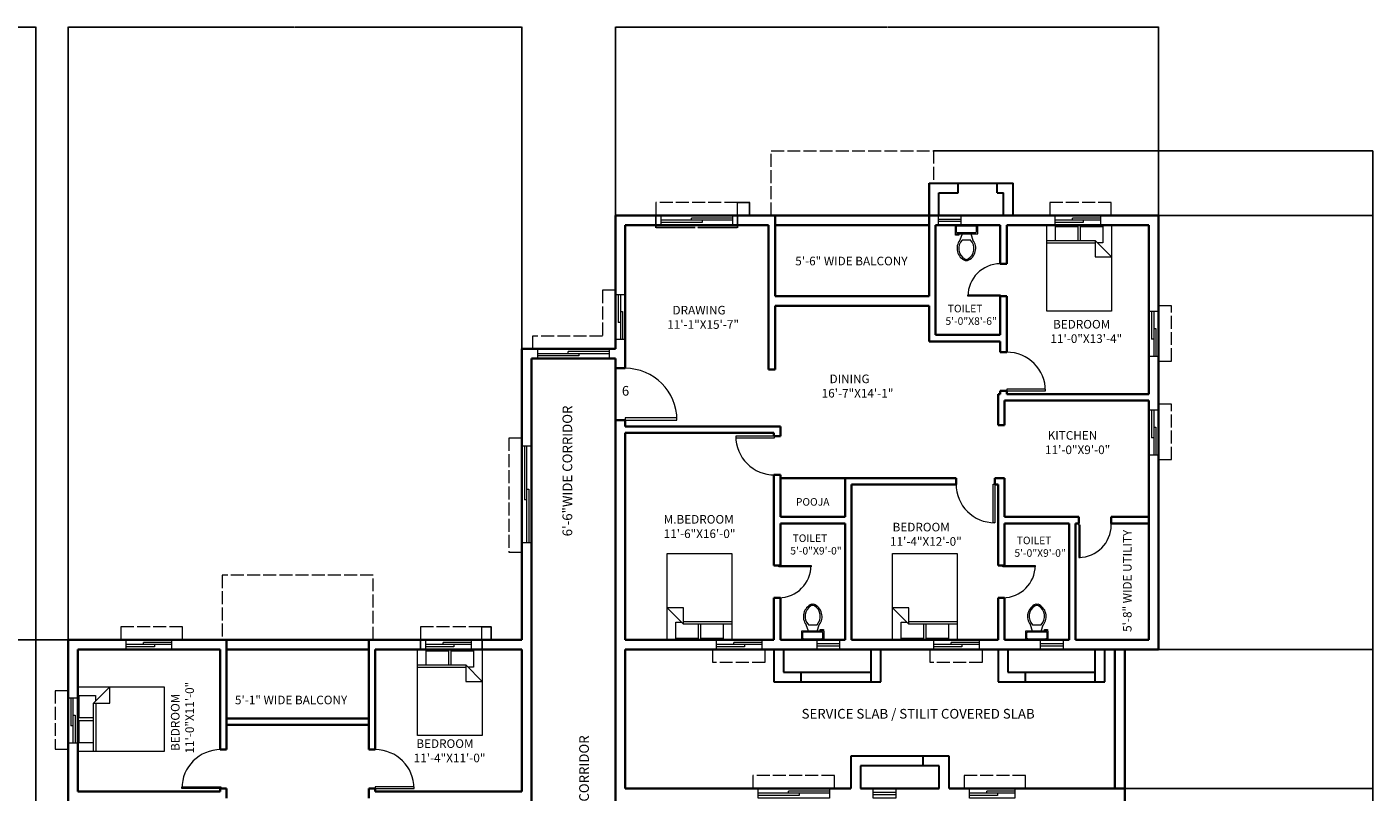
# Model space of a CAD drawing. Units: inches. Extents: x -69 to 2453, y 4803 to 7122.
# Tile 9 of 9: x 1203 to 2453, y 6411 to 7122. Entities that reach past the tile are written whole.
import ezdxf

# ---------------------------------------------------------------- set-up
doc = ezdxf.new("R2010")
doc.units = ezdxf.units.IN
doc.linetypes.add('ACAD_ISO02W100', pattern=[15, 12, -3])
for name, color, linetype, lineweight in [('A-ANNO-DIMS', 2, 'Continuous', 18), ('A-ANNO-IDEN', 2, 'Continuous', 18), ('A-AREA-IDEN', 7, 'Continuous', 18), ('A-DOOR', 3, 'Continuous', 18), ('A-FLOR-FIXT', 9, 'Continuous', 18), ('A-FLOR-OVHD', 8, 'ACAD_ISO02W100', 13), ('A-FURN', 8, 'Continuous', 18), ('A-GLAZ', 244, 'Continuous', 18), ('A-WALL', 7, 'Continuous', 35), ('A-WALL-SRVC', 7, 'Continuous', 30)]:
    doc.layers.add(name, color=color, linetype=linetype, lineweight=lineweight)
doc.styles.get("Standard").update_dxf_attribs({"font": 'arial.ttf'})
doc.dimstyles.get("Standard").update_dxf_attribs({"dimtxt": 0.18, "dimasz": 0.18, "dimexe": 0.18, "dimexo": 0.0625, "dimgap": 0.09, "dimtad": 0, "dimtih": 1, "dimtoh": 1, "dimdec": 4, "dimzin": 0, "dimdsep": 46, "dimtxsty": 'Standard', "dimcen": 0.09, "dimadec": 0, "dimazin": 0, "dimtfac": 1, "dimtdec": 4, "dimtofl": 0, "dimtmove": 0, "dimatfit": 3, "dimfxl": 1, "dimtolj": 1, "dimtzin": 0, "dimarcsym": 0})

# ---------------------------------------------------------------- blocks, each defined once
blk = doc.blocks.new('*U10')
for p, q in [((0, 0), (0, -6)), ((-40, 0), (-40, -6))]:
    blk.add_line(p, q)
blk.add_lwpolyline([(0, 0), (0, 40), (-1.75, 40), (-1.75, 0)], close=True)
blk.add_arc((0, 0), 40, 90, 180)
blk = doc.blocks.new('*U11')
for p, q in [((-40, 0), (-40, 6)), ((0, 0), (0, 6))]:
    blk.add_line(p, q)
blk.add_lwpolyline([(0, 0), (0, -40), (-1.75, -40), (-1.75, 0)], close=True)
blk.add_arc((0, 0), 40, 180, 270)
blk = doc.blocks.new('*U12')
for p, q in [((-40, 0), (-40, -6)), ((0, 0), (0, -6))]:
    blk.add_line(p, q)
blk.add_lwpolyline([(0, 0), (0, 40), (-1.75, 40), (-1.75, 0)], close=True)
blk.add_arc((0, 0), 40, 90, 180)
blk = doc.blocks.new('*U15')
for p, q in [((0, 0), (0, 6)), ((40, 0), (40, 6))]:
    blk.add_line(p, q)
blk.add_lwpolyline([(0, 0), (0, -40), (1.75, -40), (1.75, 0)], close=True)
blk.add_arc((0, 0), 40, 270, 0)
blk = doc.blocks.new('*U13')
for p, q in [((0, 0), (0, -6)), ((40, 0), (40, -6))]:
    blk.add_line(p, q)
blk.add_lwpolyline([(0, 0), (0, 40), (1.75, 40), (1.75, 0)], close=True)
blk.add_arc((0, 0), 40, 0, 90)
blk = doc.blocks.new('*U14')
for p, q in [((0, 0), (0, -6)), ((-40, 0), (-40, -6))]:
    blk.add_line(p, q)
blk.add_lwpolyline([(0, 0), (0, 40), (-1.75, 40), (-1.75, 0)], close=True)
blk.add_arc((0, 0), 40, 90, 180)
blk = doc.blocks.new('Bed - Queen')
for p, q in [((0, -80.00003), (0, 0)), ((0, 0), (59.99999, 0)), ((59.99999, 0), (59.99999, -80.00003)), ((7.99999, -1.2), (28.79998, -1.2)), ((7.99999, -14.4), (7.99999, -1.2)), ((28.79998, -1.2), (28.79998, -14.4)), ((31.19999, -1.2), (51.99999, -1.2)), ((31.19999, -14.4), (31.19999, -1.2)), ((51.99999, -1.2), (51.99999, -16.4)), ((0, -14.4), (44.8, -14.4)), ((44.8, -16.8), (0, -16.8)), ((59.99999, -29.6), (44.8, -14.4)), ((44.8, -14.4), (44.8, -29.6)), ((51.99999, -16.4), (46.79936, -16.4)), ((44.8, -29.6), (59.99999, -29.6)), ((59.99999, -80.00003), (0, -80.00003))]:
    blk.add_line(p, q)
blk = doc.blocks.new('*U33')
for p, q in [((-10, -8.5), (-8, -8.5)), ((-10, -9.5), (-10, -8.5)), ((-7, -9.5), (-10, -9.5)), ((-8, -8.5), (-8, -8)), ((-7, -8), (-7, -9.5)), ((-4, -8), (-6, -14)), ((4, -8), (6, -14)), ((9.5, -6), (9.5, -2)), ((4, -14), (-4, -14))]:
    blk.add_line(p, q)
blk.add_lwpolyline([(10.5, -8), (10.5, 0), (-10.5, 0), (-10.5, -8)], close=True)
for points in [[(-9.5, -2), (-9.5, -6)], [(8.5, -1), (-8.5, -1)], [(-8.5, -7), (8.5, -7)]]:
    blk.add_lwpolyline(points)
for centre, radius, start, end in [((-8.6, -1.9), 0.884, 81.8699, 188.1301), ((-8.6, -6.1), 0.884, 171.8699, 278.1301), ((8.6, -1.9), 0.884, 351.8699, 98.1301), ((8.6, -6.1), 0.884, 261.8699, 8.1301), ((3.5, -21.6), 12.2, 141.4691, 247.9714), ((4.2, -21.8), 11.3, 136.3677, 238.9468), ((-3.5, -21.6), 12.2, 292.0284, 38.5307), ((-4.2, -21.8), 11.3, 301.053, 43.6321), ((0, -27.9), 4, 245.7318, 294.2682), ((0, -29), 4, 254.8605, 285.1395)]:
    blk.add_arc(centre, radius, start, end)
blk = doc.blocks.new('WINDOW-VENT-21IN')
for p, q in [((0, 5.5), (21, 5.5)), ((0, 3.5), (21, 3.5))]:
    blk.add_line(p, q)
blk.add_lwpolyline([(0, 9), (21, 9), (21, 0), (0, 0)], close=True)
blk = doc.blocks.new('WINDOW-SLIDING-42IN')
for p, q in [((2.5, 42), (2.5, 16)), ((4.5, 42), (4.5, 0)), ((4.5, 26), (6.5, 26)), ((6.5, 26), (6.5, 0)), ((4.5, 16), (2.5, 16))]:
    blk.add_line(p, q)
blk.add_lwpolyline([(0, 42), (9, 42), (9, 0), (0, 0)], close=True)
blk = doc.blocks.new('WINDOW-SLIDING-66IN')
for p, q in [((66, 4.5), (0, 4.5)), ((38, 2.5), (0, 2.5)), ((66, 6.5), (28, 6.5)), ((28, 4.5), (28, 6.5)), ((38, 4.5), (38, 2.5))]:
    blk.add_line(p, q)
blk.add_lwpolyline([(66, 9), (66, 0), (0, 0), (0, 9)], close=True)
blk = doc.blocks.new('SUNSHADE-54IN')
for p, q in [((12, 54.3), (0, 54.3)), ((0, 54.3), (0, 0)), ((0, 0), (12, 0))]:
    blk.add_line(p, q)
blk = doc.blocks.new('SUNSHADE-48IN')
for p, q in [((0, 0), (0, 12)), ((48.4, 0), (0, 0)), ((48.4, 12), (48.4, 0))]:
    blk.add_line(p, q)
blk = doc.blocks.new('SUNSHADE-57IN')
for p, q in [((57.1, 12), (0, 12)), ((0, 12), (0, 0)), ((57.1, 0), (57.1, 12))]:
    blk.add_line(p, q)
blk = doc.blocks.new('SUNSHADE-51IN')
for p, q in [((12, 51.4), (0, 51.4)), ((12, 0), (12, 51.4)), ((0, 0), (12, 0))]:
    blk.add_line(p, q)
blk = doc.blocks.new('SUNSHADE-76IN')
for p, q in [((75.7, 12), (0, 12)), ((0, 12), (0, 0)), ((75.7, 0), (75.7, 12))]:
    blk.add_line(p, q)
blk = doc.blocks.new('SERVICE-BAY-78IN')
for p, q in [((0, 30), (78.1, 30)), ((0, 0), (0, 30)), ((27.1, 21), (27.1, 30)), ((63.1, 21), (63.1, 30)), ((78.1, 0), (78.1, 30)), ((9, 0), (9, 21)), ((9, 21), (27.1, 21)), ((63.1, 21), (69.1, 21)), ((69.1, 0), (69.1, 21))]:
    blk.add_line(p, q)
blk = doc.blocks.new('SERVICE-BAY-99IN')
for p, q in [((0, 30), (0, 0)), ((9, 30), (9, 9)), ((90.1, 0), (90.1, 30)), ((99.1, 0), (99.1, 30)), ((0, 0), (99.1, 0)), ((9, 9), (90.1, 9)), ((25.4, 0), (25.4, 9))]:
    blk.add_line(p, q)
blk = doc.blocks.new('*D61')
at = {"layer": 'A-ANNO-DIMS', "color": 0, "lineweight": -2, "transparency": 16777216}
for p, q in [((1568.4, 6552.7), (1568.4, 6544)), ((1625.6, 6552.7), (1625.6, 6544)), ((1568.6, 6544.1), (1595.7, 6544.1)), ((1625.4, 6544.1), (1598.3, 6544.1))]:
    blk.add_line(p, q, dxfattribs=at)
at = {"layer": 'A-ANNO-DIMS', "color": 0, "transparency": 16777216}
for points in [[(1568.6, 6544.2), (1568.6, 6544.1), (1568.4, 6544.1)], [(1625.4, 6544.2), (1625.4, 6544.1), (1625.6, 6544.1)]]:
    blk.add_solid(points, dxfattribs=at)
at = {"layer": 'Defpoints', "color": 0, "transparency": 16777216}
for p in [(1568.4, 6552.7), (1625.6, 6552.7), (1625.6, 6544.1)]:
    blk.add_point(p, dxfattribs=at)
at = {"layer": 'A-ANNO-DIMS', "color": 0, "transparency": 16777216, "insert": (1597, 6544.1), "char_height": 0.18, "attachment_point": 5}
blk.add_mtext('\\A1;SUNSHADE 57 TYP.', dxfattribs=at)
blk = doc.blocks.new('*D62')
at = {"layer": 'A-ANNO-DIMS', "color": 0, "lineweight": -2, "transparency": 16777216}
for p, q in [((1625.6, 6564.7), (1634.3, 6564.7)), ((1634.1, 6564.5), (1634.1, 6558.9)), ((1625.6, 6552.7), (1634.3, 6552.7)), ((1634.1, 6552.9), (1634.1, 6558.5))]:
    blk.add_line(p, q, dxfattribs=at)
at = {"layer": 'A-ANNO-DIMS', "color": 0, "transparency": 16777216}
for points in [[(1634.1, 6564.5), (1634.2, 6564.5), (1634.1, 6564.7)], [(1634.1, 6552.9), (1634.2, 6552.9), (1634.1, 6552.7)]]:
    blk.add_solid(points, dxfattribs=at)
at = {"layer": 'Defpoints', "color": 0, "transparency": 16777216}
for p in [(1625.6, 6564.7), (1634.1, 6564.7), (1625.6, 6552.7)]:
    blk.add_point(p, dxfattribs=at)
at = {"layer": 'A-ANNO-DIMS', "color": 0, "transparency": 16777216, "insert": (1634.1, 6558.7), "char_height": 0.18, "attachment_point": 5}
blk.add_mtext('\\A1;12 TYP.', dxfattribs=at)
blk = doc.blocks.new('*D63')
at = {"layer": 'A-ANNO-DIMS', "color": 0, "lineweight": -2, "transparency": 16777216}
for p, q in [((1786.9, 6946.7), (1786.9, 6935.2)), ((1862.6, 6946.7), (1862.6, 6935.2)), ((1787.1, 6935.4), (1823.5, 6935.4)), ((1862.4, 6935.4), (1826, 6935.4))]:
    blk.add_line(p, q, dxfattribs=at)
at = {"layer": 'A-ANNO-DIMS', "color": 0, "transparency": 16777216}
for points in [[(1787.1, 6935.4), (1787.1, 6935.3), (1786.9, 6935.4)], [(1862.4, 6935.4), (1862.4, 6935.3), (1862.6, 6935.4)]]:
    blk.add_solid(points, dxfattribs=at)
at = {"layer": 'Defpoints', "color": 0, "transparency": 16777216}
for p in [(1786.9, 6946.7), (1862.6, 6946.7), (1862.6, 6935.4)]:
    blk.add_point(p, dxfattribs=at)
at = {"layer": 'A-ANNO-DIMS', "color": 0, "transparency": 16777216, "insert": (1824.8, 6935.4), "char_height": 0.18, "attachment_point": 5}
blk.add_mtext('\\A1;SUNSHADE 76 TYP.', dxfattribs=at)
blk = doc.blocks.new('*D64')
at = {"layer": 'A-ANNO-DIMS', "color": 0, "lineweight": -2, "transparency": 16777216}
for p, q in [((1862.7, 6958.7), (1874.1, 6958.7)), ((1873.9, 6958.5), (1873.9, 6952.9)), ((1862.7, 6946.7), (1874.1, 6946.7)), ((1873.9, 6946.9), (1873.9, 6952.5))]:
    blk.add_line(p, q, dxfattribs=at)
at = {"layer": 'A-ANNO-DIMS', "color": 0, "transparency": 16777216}
for points in [[(1873.9, 6958.5), (1874, 6958.5), (1873.9, 6958.7)], [(1873.9, 6946.9), (1874, 6946.9), (1873.9, 6946.7)]]:
    blk.add_solid(points, dxfattribs=at)
at = {"layer": 'Defpoints', "color": 0, "transparency": 16777216}
for p in [(1862.6, 6958.7), (1873.9, 6958.7), (1862.6, 6946.7)]:
    blk.add_point(p, dxfattribs=at)
at = {"layer": 'A-ANNO-DIMS', "color": 0, "transparency": 16777216, "insert": (1873.9, 6952.7), "char_height": 0.18, "attachment_point": 5}
blk.add_mtext('\\A1;12 TYP.', dxfattribs=at)
blk = doc.blocks.new('*D92')
at = {"layer": 'A-ANNO-DIMS', "color": 0, "lineweight": -2, "transparency": 16777216}
for p, q in [((2222.1, 6414.7), (2452.4, 6414.7)), ((2452.3, 6414.5), (2452.3, 6221.4)), ((2452.3, 6027.9), (2452.3, 6221)), ((2222.1, 6027.7), (2452.4, 6027.7))]:
    blk.add_line(p, q, dxfattribs=at)
at = {"layer": 'A-ANNO-DIMS', "color": 0, "transparency": 16777216}
for points in [[(2452.2, 6414.5), (2452.3, 6414.5), (2452.3, 6414.7)], [(2452.2, 6027.9), (2452.3, 6027.9), (2452.3, 6027.7)]]:
    blk.add_solid(points, dxfattribs=at)
at = {"layer": 'Defpoints', "color": 0, "transparency": 16777216}
for p in [(2222, 6414.7), (2452.3, 6414.7), (2222, 6027.7)]:
    blk.add_point(p, dxfattribs=at)
at = {"layer": 'A-ANNO-DIMS', "color": 0, "transparency": 16777216, "insert": (2452.3, 6221.2), "char_height": 0.18, "attachment_point": 5}
blk.add_mtext('\\A1;387', dxfattribs=at)
blk = doc.blocks.new('*D93')
at = {"layer": 'A-ANNO-DIMS', "color": 0, "lineweight": -2, "transparency": 16777216}
for p, q in [((2253.6, 6543.7), (2452.4, 6543.7)), ((2452.3, 6543.5), (2452.3, 6479.4)), ((2452.3, 6414.9), (2452.3, 6479)), ((2222.1, 6414.7), (2452.4, 6414.7))]:
    blk.add_line(p, q, dxfattribs=at)
at = {"layer": 'A-ANNO-DIMS', "color": 0, "transparency": 16777216}
for points in [[(2452.2, 6543.5), (2452.3, 6543.5), (2452.3, 6543.7)], [(2452.2, 6414.9), (2452.3, 6414.9), (2452.3, 6414.7)]]:
    blk.add_solid(points, dxfattribs=at)
at = {"layer": 'Defpoints', "color": 0, "transparency": 16777216}
for p in [(2253.5, 6543.7), (2452.3, 6543.7), (2222, 6414.7)]:
    blk.add_point(p, dxfattribs=at)
at = {"layer": 'A-ANNO-DIMS', "color": 0, "transparency": 16777216, "insert": (2452.3, 6479.2), "char_height": 0.18, "attachment_point": 5}
blk.add_mtext('\\A1;129', dxfattribs=at)
blk = doc.blocks.new('*D94')
at = {"layer": 'A-ANNO-DIMS', "color": 0, "lineweight": -2, "transparency": 16777216}
for p, q in [((2253.6, 6946.7), (2452.4, 6946.7)), ((2452.3, 6946.5), (2452.3, 6745.4)), ((2452.3, 6543.9), (2452.3, 6745)), ((2253.6, 6543.7), (2452.4, 6543.7))]:
    blk.add_line(p, q, dxfattribs=at)
at = {"layer": 'A-ANNO-DIMS', "color": 0, "transparency": 16777216}
for points in [[(2452.2, 6946.5), (2452.3, 6946.5), (2452.3, 6946.7)], [(2452.2, 6543.9), (2452.3, 6543.9), (2452.3, 6543.7)]]:
    blk.add_solid(points, dxfattribs=at)
at = {"layer": 'Defpoints', "color": 0, "transparency": 16777216}
for p in [(2253.5, 6946.7), (2452.3, 6946.7), (2253.5, 6543.7)]:
    blk.add_point(p, dxfattribs=at)
at = {"layer": 'A-ANNO-DIMS', "color": 0, "transparency": 16777216, "insert": (2452.3, 6745.2), "char_height": 0.18, "attachment_point": 5}
blk.add_mtext('\\A1;403', dxfattribs=at)
blk = doc.blocks.new('*D96')
at = {"layer": 'A-ANNO-DIMS', "color": 0, "lineweight": -2, "transparency": 16777216}
for p, q in [((2044.6, 7006.7), (2452.4, 7006.7)), ((2452.3, 7006.5), (2452.3, 5962.4)), ((2452.3, 4917.9), (2452.3, 5962)), ((2143.1, 4917.7), (2452.4, 4917.7))]:
    blk.add_line(p, q, dxfattribs=at)
at = {"layer": 'A-ANNO-DIMS', "color": 0, "transparency": 16777216}
for points in [[(2452.2, 7006.5), (2452.3, 7006.5), (2452.3, 7006.7)], [(2452.2, 4917.9), (2452.3, 4917.9), (2452.3, 4917.7)]]:
    blk.add_solid(points, dxfattribs=at)
at = {"layer": 'Defpoints', "color": 0, "transparency": 16777216}
for p in [(2044.6, 7006.7), (2452.3, 7006.7), (2143.1, 4917.7)]:
    blk.add_point(p, dxfattribs=at)
at = {"layer": 'A-ANNO-DIMS', "color": 0, "transparency": 16777216, "insert": (2452.3, 5962.2), "char_height": 0.18, "attachment_point": 5}
blk.add_mtext('\\A1;2089', dxfattribs=at)
blk = doc.blocks.new('*D100')
at = {"layer": 'A-ANNO-DIMS', "color": 0, "lineweight": -2, "transparency": 16777216}
for p, q in [((752.5, 6159.8), (752.5, 7121.6)), ((752.7, 7121.5), (981.7, 7121.5)), ((1211.3, 7121.5), (982.3, 7121.5)), ((1211.5, 6159.8), (1211.5, 7121.6))]:
    blk.add_line(p, q, dxfattribs=at)
at = {"layer": 'A-ANNO-DIMS', "color": 0, "transparency": 16777216}
for points in [[(752.7, 7121.5), (752.7, 7121.4), (752.5, 7121.5)], [(1211.3, 7121.5), (1211.3, 7121.4), (1211.5, 7121.5)]]:
    blk.add_solid(points, dxfattribs=at)
at = {"layer": 'Defpoints', "color": 0, "transparency": 16777216}
for p in [(1211.5, 7121.5), (752.5, 6159.7), (1211.5, 6159.7)]:
    blk.add_point(p, dxfattribs=at)
at = {"layer": 'A-ANNO-DIMS', "color": 0, "transparency": 16777216, "insert": (982, 7121.5), "char_height": 0.18, "attachment_point": 5}
blk.add_mtext('\\A1;459', dxfattribs=at)
blk = doc.blocks.new('*D102')
at = {"layer": 'A-ANNO-DIMS', "color": 0, "lineweight": -2, "transparency": 16777216}
for p, q in [((1241.5, 6552.8), (1241.5, 7121.6)), ((1241.7, 7121.5), (1451.7, 7121.5)), ((1662.3, 7121.5), (1452.3, 7121.5)), ((1662.5, 6552.8), (1662.5, 7121.6))]:
    blk.add_line(p, q, dxfattribs=at)
at = {"layer": 'A-ANNO-DIMS', "color": 0, "transparency": 16777216}
for points in [[(1241.7, 7121.5), (1241.7, 7121.4), (1241.5, 7121.5)], [(1662.3, 7121.5), (1662.3, 7121.4), (1662.5, 7121.5)]]:
    blk.add_solid(points, dxfattribs=at)
at = {"layer": 'Defpoints', "color": 0, "transparency": 16777216}
for p in [(1662.5, 7121.5), (1241.5, 6552.7), (1662.5, 6552.7)]:
    blk.add_point(p, dxfattribs=at)
at = {"layer": 'A-ANNO-DIMS', "color": 0, "transparency": 16777216, "insert": (1452, 7121.5), "char_height": 0.18, "attachment_point": 5}
blk.add_mtext('\\A1;421', dxfattribs=at)
blk = doc.blocks.new('*D103')
at = {"layer": 'A-ANNO-DIMS', "color": 0, "lineweight": -2, "transparency": 16777216}
for p, q in [((1241.4, 6552.7), (-69.4, 6552.7)), ((-69.2, 6552.5), (-69.2, 6345.9)), ((-69.2, 6138.9), (-69.2, 6345.5)), ((1241.4, 6138.7), (-69.4, 6138.7))]:
    blk.add_line(p, q, dxfattribs=at)
at = {"layer": 'A-ANNO-DIMS', "color": 0, "transparency": 16777216}
for points in [[(-69.3, 6552.5), (-69.2, 6552.5), (-69.2, 6552.7)], [(-69.3, 6138.9), (-69.2, 6138.9), (-69.2, 6138.7)]]:
    blk.add_solid(points, dxfattribs=at)
at = {"layer": 'Defpoints', "color": 0, "transparency": 16777216}
for p in [(-69.2, 6552.7), (1241.5, 6552.7), (1241.5, 6138.7)]:
    blk.add_point(p, dxfattribs=at)
at = {"layer": 'A-ANNO-DIMS', "color": 0, "transparency": 16777216, "insert": (-69.2, 6345.7), "char_height": 0.18, "attachment_point": 5}
blk.add_mtext('\\A1;414', dxfattribs=at)
blk = doc.blocks.new('*D104')
at = {"layer": 'A-ANNO-DIMS', "color": 0, "lineweight": -2, "transparency": 16777216}
for p, q in [((1749.5, 6946.8), (1749.5, 7121.6)), ((1749.7, 7121.5), (2001.2, 7121.5)), ((2253.3, 7121.5), (2001.8, 7121.5)), ((2253.5, 6946.8), (2253.5, 7121.6))]:
    blk.add_line(p, q, dxfattribs=at)
at = {"layer": 'A-ANNO-DIMS', "color": 0, "transparency": 16777216}
for points in [[(1749.7, 7121.5), (1749.7, 7121.4), (1749.5, 7121.5)], [(2253.3, 7121.5), (2253.3, 7121.4), (2253.5, 7121.5)]]:
    blk.add_solid(points, dxfattribs=at)
at = {"layer": 'Defpoints', "color": 0, "transparency": 16777216}
for p in [(2253.5, 7121.5), (1749.5, 6946.7), (2253.5, 6946.7)]:
    blk.add_point(p, dxfattribs=at)
at = {"layer": 'A-ANNO-DIMS', "color": 0, "transparency": 16777216, "insert": (2001.5, 7121.5), "char_height": 0.18, "attachment_point": 5}
blk.add_mtext('\\A1;504', dxfattribs=at)

msp = doc.modelspace()

# ---------------------------------------------------------------- linework, layer by layer
at = {"layer": 'A-FLOR-OVHD'}
for p, q in [((1894, 6946.7), (1894, 7006.7)), ((1894, 7006.7), (2044.6, 7006.7)), ((2044.6, 7006.7), (2044.6, 6976.7)), ((1749.5, 6877.1), (1737.5, 6877.1)), ((1737.5, 6877.1), (1737.5, 6834.7)), ((1737.5, 6834.7), (1672.4, 6834.7)), ((1672.4, 6834.7), (1672.4, 6822.7)), ((1662.5, 6740), (1650.5, 6740)), ((1650.5, 6740), (1650.5, 6634)), ((1650.5, 6634), (1662.5, 6634)), ((1524.6, 6612.7), (1384.3, 6612.7)), ((1384.3, 6612.7), (1384.3, 6552.7)), ((1524.6, 6552.7), (1524.6, 6612.7))]:
    msp.add_line(p, q, dxfattribs=at)
at = {"layer": 'A-GLAZ'}
for p, q in [((1665, 6732.6), (1665, 6682.6)), ((1667, 6732.6), (1667, 6642.6)), ((1667, 6692.6), (1669, 6692.6)), ((1669, 6692.6), (1669, 6642.6)), ((1667, 6682.6), (1665, 6682.6))]:
    msp.add_line(p, q, dxfattribs=at)
msp.add_lwpolyline([(1662.5, 6732.6), (1671.5, 6732.6), (1671.5, 6642.6), (1662.5, 6642.6)], close=True, dxfattribs=at)
at = {"layer": 'A-WALL'}
for p, q in [((2040.5, 6871.7), (2040.5, 6976.7)), ((1749.5, 6946.7), (2253.5, 6946.7)), ((1749.5, 6822.7), (1749.5, 6946.7)), ((1897.5, 6871.7), (1897.5, 6946.7)), ((2253.5, 6543.7), (2253.5, 6946.7)), ((1758.5, 6937.7), (1891.5, 6937.7)), ((1758.5, 6804.7), (1758.5, 6937.7)), ((1891.5, 6937.7), (1891.5, 6803.7)), ((1897.5, 6937.7), (2040.5, 6937.7)), ((2046.5, 6835.7), (2046.5, 6937.7)), ((2046.5, 6937.7), (2106.5, 6937.7)), ((2106.5, 6901.7), (2106.5, 6937.7)), ((2112.5, 6937.7), (2244.5, 6937.7)), ((2112.5, 6901.7), (2112.5, 6937.7)), ((2244.5, 6780.7), (2244.5, 6937.7)), ((2106.5, 6901.7), (2112.5, 6901.7)), ((1897.5, 6871.7), (2040.5, 6871.7)), ((2106.5, 6835.7), (2106.5, 6871.7)), ((2106.5, 6871.7), (2112.5, 6871.7)), ((2112.5, 6819.7), (2112.5, 6871.7)), ((1897.5, 6862.7), (2040.5, 6862.7)), ((1897.5, 6862.7), (1897.5, 6803.7)), ((2040.5, 6829.7), (2040.5, 6862.7)), ((2046.5, 6835.7), (2106.5, 6835.7)), ((1749.5, 6822.7), (1662.5, 6822.7)), ((1662.5, 6552.7), (1662.5, 6822.7)), ((2040.5, 6829.7), (2106.5, 6829.7)), ((2106.5, 6819.7), (2106.5, 6829.7)), ((1671.5, 6212.2), (1671.5, 6813.7)), ((1749.5, 6813.7), (1671.5, 6813.7)), ((1749.5, 6308.2), (1749.5, 6813.7)), ((2112.5, 6819.7), (2106.5, 6819.7)), ((1758.5, 6804.7), (1749.5, 6804.7)), ((1891.5, 6803.7), (1897.5, 6803.7)), ((2106.5, 6780.7), (2106.5, 6783.7)), ((2112.5, 6783.7), (2106.5, 6783.7)), ((2112.5, 6780.7), (2112.5, 6783.7)), ((2104.5, 6780.7), (2106.5, 6780.7)), ((2104.5, 6780.7), (2104.5, 6752)), ((2110.5, 6774.7), (2244.5, 6774.7)), ((2110.5, 6752), (2110.5, 6774.7)), ((2112.5, 6780.7), (2244.5, 6780.7)), ((2244.5, 6552.7), (2244.5, 6774.7)), ((1758.5, 6756.7), (1749.5, 6756.7)), ((1758.5, 6750.7), (1758.5, 6756.7)), ((1758.5, 6750.7), (1902.5, 6750.7)), ((1902.5, 6741.7), (1902.5, 6750.7)), ((2110.5, 6752), (2104.5, 6752)), ((1758.5, 6744.7), (1896.5, 6744.7)), ((1758.5, 6552.7), (1758.5, 6744.7)), ((1896.5, 6741.7), (1896.5, 6744.7)), ((1896.5, 6741.7), (1902.5, 6741.7)), ((1896.5, 6705.7), (1902.5, 6705.7)), ((1896.5, 6621.7), (1896.5, 6705.7)), ((1902.5, 6666.7), (1902.5, 6705.7)), ((1902.5, 6702.7), (2065.5, 6702.7)), ((1962.5, 6666.7), (1962.5, 6702.7)), ((1968.5, 6552.7), (1968.5, 6696.7)), ((1968.5, 6696.7), (2065.5, 6696.7)), ((2065.5, 6696.7), (2065.5, 6702.7)), ((2101.5, 6696.7), (2101.5, 6702.7)), ((2101.5, 6702.7), (2110.5, 6702.7)), ((2101.5, 6696.7), (2104.5, 6696.7)), ((2104.5, 6621.7), (2104.5, 6696.7)), ((2110.5, 6666.7), (2110.5, 6702.7)), ((1902.5, 6666.7), (1962.5, 6666.7)), ((1902.5, 6660.7), (1962.5, 6660.7)), ((1902.5, 6621.7), (1902.5, 6660.7)), ((1962.5, 6552.7), (1962.5, 6660.7)), ((2110.5, 6666.7), (2179.5, 6666.7)), ((2110.5, 6660.7), (2170.5, 6660.7)), ((2110.5, 6621.7), (2110.5, 6660.7)), ((2170.5, 6552.7), (2170.5, 6660.7)), ((2176.5, 6552.7), (2176.5, 6660.7)), ((2176.5, 6660.7), (2179.5, 6660.7)), ((2179.5, 6660.7), (2179.5, 6666.7)), ((2209.5, 6660.7), (2209.5, 6666.7)), ((2209.5, 6666.7), (2244.5, 6666.7)), ((2209.5, 6660.7), (2244.5, 6660.7)), ((1902.5, 6621.7), (1896.5, 6621.7)), ((2110.5, 6621.7), (2104.5, 6621.7)), ((1896.5, 6552.7), (1896.5, 6591.7)), ((1902.5, 6591.7), (1896.5, 6591.7)), ((1902.5, 6552.7), (1902.5, 6591.7)), ((2104.5, 6552.7), (2104.5, 6591.7)), ((2110.5, 6591.7), (2104.5, 6591.7)), ((2110.5, 6552.7), (2110.5, 6591.7)), ((1241.5, 6138.7), (1241.5, 6552.7)), ((1241.5, 6552.7), (1662.5, 6552.7)), ((1388.5, 6450.7), (1388.5, 6552.7)), ((1520.5, 6450.7), (1520.5, 6552.7)), ((1758.5, 6552.7), (1896.5, 6552.7)), ((1902.5, 6552.7), (1962.5, 6552.7)), ((1968.5, 6552.7), (2104.5, 6552.7)), ((2110.5, 6552.7), (2170.5, 6552.7)), ((2176.5, 6552.7), (2244.5, 6552.7)), ((1250.5, 6543.7), (1382.5, 6543.7)), ((1250.5, 6411.7), (1250.5, 6543.7)), ((1382.5, 6450.7), (1382.5, 6543.7)), ((1388.5, 6543.7), (1520.5, 6543.7)), ((1526.5, 6543.7), (1662.5, 6543.7)), ((1526.5, 6450.7), (1526.5, 6543.7)), ((1662.5, 6411.7), (1662.5, 6543.7)), ((1758.5, 6543.7), (2253.5, 6543.7)), ((1758.5, 6414.7), (1758.5, 6543.7)), ((2213, 6543.7), (2213, 6414.7)), ((2222, 6543.7), (2222, 5382.7)), ((1388.5, 6479.7), (1520.5, 6479.7)), ((1388.5, 6473.7), (1520.5, 6473.7)), ((1382.5, 6450.7), (1388.5, 6450.7)), ((1526.5, 6450.7), (1520.5, 6450.7)), ((1250.5, 6411.7), (1382.5, 6411.7)), ((1382.5, 6411.7), (1382.5, 6414.7)), ((1382.5, 6414.7), (1388.5, 6414.7)), ((1388.5, 6405.7), (1388.5, 6414.7)), ((1520.5, 6405.7), (1520.5, 6414.7)), ((1526.5, 6414.7), (1520.5, 6414.7)), ((1526.5, 6411.7), (1526.5, 6414.7)), ((1526.5, 6411.7), (1662.5, 6411.7)), ((1758.5, 6414.7), (1967.9, 6414.7)), ((1976.9, 6414.7), (2050, 6414.7)), ((2059, 6414.7), (2222, 6414.7))]:
    msp.add_line(p, q, dxfattribs=at)
at = {"layer": 'A-WALL-SRVC'}
for p, q in [((1967.9, 6444.7), (1967.9, 6414.7)), ((2059, 6444.7), (1967.9, 6444.7)), ((2050, 6435.7), (1976.9, 6435.7)), ((1976.9, 6435.7), (1976.9, 6414.7)), ((2034.9, 6435.7), (2034.9, 6444.7)), ((2050, 6414.7), (2050, 6435.7)), ((2059, 6414.7), (2059, 6444.7))]:
    msp.add_line(p, q, dxfattribs=at)

# ---------------------------------------------------------------- block references
at = {"layer": 'A-DOOR'}
for name, p, xscale, yscale, zscale, rotation in [('*U11', (2106.5, 6871.7), 0.75, 0.75, 0.75, 270.0000000000001), ('*U10', (2112.5, 6783.7), 0.9, 0.9, 0.9, 270), ('*U12', (1758.5, 6756.7), 1.199999999999977, 1.199999999999977, 1.199999999999977, 270.0000000000001), ('*U15', (1897.1, 6741.7), 0.9, 0.9, 0.9, 270), ('*U14', (2179.5, 6659.2), 0.75, 0.75, 0.75, 180), ('*U13', (1901, 6621.7), 0.75, 0.75, 0.75, 270.0000000000001), ('*U13', (2109, 6621.7), 0.75, 0.75, 0.75, 270.0000000000001), ('*U11', (1383.1, 6414.7), 0.9, 0.9, 0.9, 270), ('*U10', (1526.5, 6414.7), 0.9, 0.9, 0.9, 270)]:
    msp.add_blockref(name, p, dxfattribs=dict(at, xscale=xscale, yscale=yscale, zscale=zscale, rotation=rotation))
at = {"layer": 'A-DOOR', "xscale": 0.9, "yscale": 0.9, "zscale": 0.9}
msp.add_blockref('*U11', (2101.5, 6697.3), dxfattribs=at)
at = {"layer": 'A-FLOR-FIXT'}
msp.add_blockref('*U33', (2075.1, 6937.7), dxfattribs=at)
at = {"layer": 'A-FLOR-FIXT', "rotation": 180}
for p in [(1932.5, 6552.7), (2140.5, 6552.7)]:
    msp.add_blockref('*U33', p, dxfattribs=at)
at = {"layer": 'A-FLOR-OVHD'}
for name, p in [('SUNSHADE-76IN', (1786.9, 6946.7)), ('SUNSHADE-57IN', (2152.4, 6946.7)), ('SUNSHADE-51IN', (2253.5, 6811.4)), ('SUNSHADE-51IN', (2253.5, 6719.9)), ('SUNSHADE-57IN', (1290.4, 6552.7)), ('SUNSHADE-57IN', (1568.4, 6552.7)), ('SUNSHADE-48IN', (1839.8, 6531.7)), ('SUNSHADE-48IN', (2041.4, 6531.7)), ('SUNSHADE-54IN', (1229.5, 6451.1)), ('SUNSHADE-76IN', (1876.9, 6414.7)), ('SUNSHADE-57IN', (2072.9, 6414.7))]:
    msp.add_blockref(name, p, dxfattribs=at)
at = {"layer": 'A-FURN'}
for p in [(2149.7, 6937.7), (1565.7, 6543.7)]:
    msp.add_blockref('Bed - Queen', p, dxfattribs=at)
for p, rotation in [((1857.5, 6552.7), 180), ((2066.5, 6552.7), 180), ((1250.5, 6448.9), 89.99999999999999)]:
    msp.add_blockref('Bed - Queen', p, dxfattribs=dict(at, rotation=rotation))
at = {"layer": 'A-GLAZ'}
for name, p in [('WINDOW-SLIDING-66IN', (1792, 6937.7)), ('WINDOW-VENT-21IN', (2049.1, 6937.7)), ('WINDOW-SLIDING-42IN', (1749.5, 6831.3)), ('WINDOW-SLIDING-42IN', (2244.5, 6815.7)), ('WINDOW-SLIDING-66IN', (1677.5, 6813.7)), ('WINDOW-SLIDING-42IN', (2244.5, 6724.2)), ('WINDOW-VENT-21IN', (1936.5, 6543.7)), ('WINDOW-VENT-21IN', (2143.8, 6543.7)), ('WINDOW-SLIDING-42IN', (1241.5, 6456.7)), ('WINDOW-SLIDING-66IN', (1882, 6405.7)), ('WINDOW-VENT-21IN', (1988.5, 6405.7))]:
    msp.add_blockref(name, p, dxfattribs=at)
for p, rotation in [((2157.5, 6946.7), 270.0000000000031), ((1295.5, 6552.7), 270.0000000000007), ((1573.5, 6552.7), 269.9999999999984), ((1843.3, 6552.7), 269.9999999999964), ((2044.9, 6552.7), 269.9999999999985), ((2078, 6414.7), 270.0000000000009)]:
    msp.add_blockref('WINDOW-SLIDING-42IN', p, dxfattribs=dict(at, rotation=rotation))
at = {"layer": 'A-WALL-SRVC'}
for name, p in [('SERVICE-BAY-78IN', (2040.5, 6946.7)), ('SERVICE-BAY-99IN', (1896.5, 6513.7)), ('SERVICE-BAY-99IN', (2104.5, 6513.7))]:
    msp.add_blockref(name, p, dxfattribs=at)

# ---------------------------------------------------------------- texts
at = {"layer": 'A-ANNO-IDEN', "insert": (1755.4, 6788.3), "char_height": 8, "attachment_point": 1}
msp.add_mtext_dynamic_manual_height_columns('{\\H1.125x;6} ', width=10.499, gutter_width=12.5, heights=[0], dxfattribs=at)
at = {"layer": 'A-AREA-IDEN', "attachment_point": 1}
for s, width, insert, char_height in [('5\'-6" WIDE BALCONY', 114.375, (1916.3, 6908.3), 8), ('  DRAWING\\P11\'-1"X15\'-7"', 66.094, (1797.5, 6862.7), 8), (' TOILET\\P5\'-0"X8\'-6"', 45.2, (2055.7, 6863.7), 7), (' BEDROOM\\P11\'-0"X13\'-4"', 64.991, (2153.1, 6849.6), 8), ('   DINING\\P16\'-7"X14\'-1"', 63.236, (1940.8, 6798.9), 8), (' KITCHEN\\P11\'-0"X9\'-0"', 58.128, (2148.1, 6746.4), 8), ('POOJA', 33.919, (1916.9, 6684.2), 7), ('M.BEDROOM\\P11\'-6"X16\'-0"', 69.603, (1794.2, 6668.5), 8), (' BEDROOM\\P11\'-4"X12\'-0"', 64.991, (2004.2, 6661.3), 8), (' TOILET\\P5\'-0"X9\'-0"', 45.2, (1911.7, 6650.5), 7), (' TOILET\\P5\'-0"X9\'-0"', 45.2, (2119.7, 6648.4), 7), ('5\'-1" WIDE BALCONY', 114.375, (1396.3, 6500.8), 8), ('SERVICE SLAB / STILIT COVERED SLAB', 244.202, (1922.2, 6488.5), 9), (' BEDROOM\\P11\'-4"X11\'-0"', 64.991, (1562.2, 6460.3), 8)]:
    msp.add_mtext_dynamic_manual_height_columns(s, width=width, gutter_width=12.5, heights=[0], dxfattribs=dict(at, insert=insert, char_height=char_height))
at = {"layer": 'A-AREA-IDEN', "attachment_point": 1, "rotation": 90}
for s, width, insert, char_height in [('6\'-6"WIDE CORRIDOR', 131.057, (1700.3, 6648.7), 9), ('5\'-8" WIDE UTILITY', 99.552, (2220.4, 6560), 8), (' BEDROOM\\P11\'-0"X11\'-0"', 64.991, (1336.9, 6447.1), 8), ('6\'-6"WIDE CORRIDOR', 131.057, (1715.8, 6342.5), 9)]:
    msp.add_mtext_dynamic_manual_height_columns(s, width=width, gutter_width=12.5, heights=[0], dxfattribs=dict(at, insert=insert, char_height=char_height))

# ---------------------------------------------------------------- dimensions: what is measured, and where the dimension line sits
at = {"layer": 'A-ANNO-DIMS'}
for base, p1, p2, picture, middle in [((1211.5, 7121.5), (752.5, 6159.7), (1211.5, 6159.7), '*D100', (982, 7121.5)), ((1662.5, 7121.5), (1241.5, 6552.7), (1662.5, 6552.7), '*D102', (1452, 7121.5)), ((2253.5, 7121.5), (1749.5, 6946.7), (2253.5, 6946.7), '*D104', (2001.5, 7121.5))]:
    dim = msp.add_linear_dim(base=base, p1=p1, p2=p2, dimstyle='Standard', override={"dimdec": 0, "dimlfac": 1, "dimrnd": 0, "dimzin": 0, "dimdsep": 46, "dimlunit": 2}, dxfattribs=at)
    dim.commit()
    dim.dimension.update_dxf_attribs({"geometry": picture, "text_midpoint": middle})
for base, p1, p2, picture, middle in [((2452.3, 7006.7), (2143.1, 4917.7), (2044.6, 7006.7), '*D96', (2452.3, 5962.2)), ((2452.3, 6946.7), (2253.5, 6543.7), (2253.5, 6946.7), '*D94', (2452.3, 6745.2)), ((-69.2, 6552.7), (1241.5, 6138.7), (1241.5, 6552.7), '*D103', (-69.2, 6345.7)), ((2452.3, 6543.7), (2222, 6414.7), (2253.5, 6543.7), '*D93', (2452.3, 6479.2)), ((2452.3, 6414.7), (2222, 6027.7), (2222, 6414.7), '*D92', (2452.3, 6221.2))]:
    dim = msp.add_linear_dim(base=base, p1=p1, p2=p2, angle=90, dimstyle='Standard', override={"dimdec": 0, "dimlfac": 1, "dimrnd": 0, "dimzin": 0, "dimdsep": 46, "dimlunit": 2}, dxfattribs=at)
    dim.commit()
    dim.dimension.update_dxf_attribs({"geometry": picture, "text_midpoint": middle})
for base, p1, p2, picture, middle in [((1873.9, 6958.7), (1862.6, 6946.7), (1862.6, 6958.7), '*D64', (1873.9, 6952.7)), ((1634.1, 6564.7), (1625.6, 6552.7), (1625.6, 6564.7), '*D62', (1634.1, 6558.7))]:
    dim = msp.add_linear_dim(base=base, p1=p1, p2=p2, angle=90, text='<> TYP.', dimstyle='Standard', override={"dimdec": 0, "dimlfac": 1, "dimrnd": 0, "dimzin": 0, "dimdsep": 46, "dimlunit": 2}, dxfattribs=at)
    dim.commit()
    dim.dimension.update_dxf_attribs({"geometry": picture, "text_midpoint": middle})
for base, p1, p2, picture, middle in [((1862.6, 6935.4), (1786.9, 6946.7), (1862.6, 6946.7), '*D63', (1824.8, 6935.4)), ((1625.6, 6544.1), (1568.4, 6552.7), (1625.6, 6552.7), '*D61', (1597, 6544.1))]:
    dim = msp.add_linear_dim(base=base, p1=p1, p2=p2, text='SUNSHADE <> TYP.', dimstyle='Standard', override={"dimdec": 0, "dimlfac": 1, "dimrnd": 0, "dimzin": 0, "dimdsep": 46, "dimlunit": 2}, dxfattribs=at)
    dim.commit()
    dim.dimension.update_dxf_attribs({"geometry": picture, "text_midpoint": middle})

doc.saveas('drawing.dxf')
